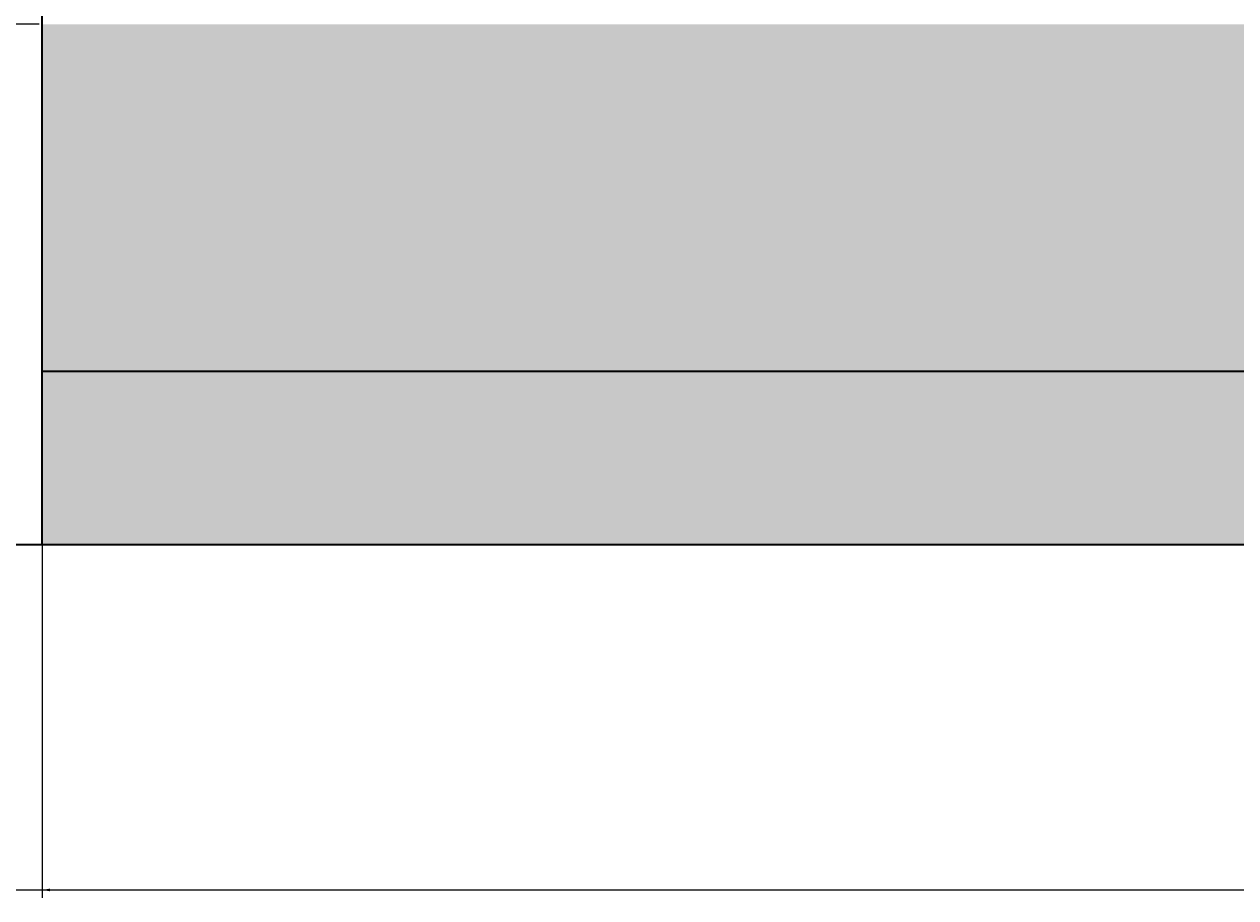
# Model space of a CAD drawing. Units: inches. Extents: x 4508 to 4723, y 847 to 1020.
# Tile 2 of 32: x 4550 to 4577, y 867 to 887. Entities that reach past the tile are written whole.
import ezdxf

# ---------------------------------------------------------------- set-up
doc = ezdxf.new("R2010")
doc.units = ezdxf.units.IN
for name, color, linetype, lineweight in [('A-ANNO-DIMS', 2, 'Continuous', 18), ('A-WALL', 7, 'Continuous', 35), ('A-WALL-PATT', 254, 'Continuous', 13)]:
    doc.layers.add(name, color=color, linetype=linetype, lineweight=lineweight)
doc.styles.get("Standard").update_dxf_attribs({"font": 'arial.ttf'})
doc.dimstyles.get("Standard").update_dxf_attribs({"dimtxt": 0.18, "dimasz": 0.18, "dimexe": 0.18, "dimexo": 0.0625, "dimgap": 0.09, "dimtad": 0, "dimtih": 1, "dimtoh": 1, "dimdec": 4, "dimzin": 0, "dimdsep": 46, "dimtxsty": 'Standard', "dimcen": 0.09, "dimadec": 0, "dimazin": 0, "dimtfac": 1, "dimtdec": 4, "dimtofl": 0, "dimtmove": 0, "dimatfit": 3, "dimfxl": 1, "dimtolj": 1, "dimtzin": 0, "dimarcsym": 0})

# ---------------------------------------------------------------- blocks, each defined once
blk = doc.blocks.new('*D2')
at = {"layer": 'A-ANNO-DIMS', "color": 0, "lineweight": -2, "transparency": 16777216}
for p, q in [((4540.994, 874.684), (4540.994, 866.617)), ((4693.994, 874.684), (4693.994, 866.617)), ((4541.174, 866.797), (4617.213, 866.797)), ((4693.814, 866.797), (4617.774, 866.797))]:
    blk.add_line(p, q, dxfattribs=at)
at = {"layer": 'A-ANNO-DIMS', "color": 0, "lineweight": 9, "transparency": 16777216}
for points in [[(4541.174, 866.827), (4541.174, 866.767), (4540.994, 866.797)], [(4693.814, 866.827), (4693.814, 866.767), (4693.994, 866.797)]]:
    blk.add_solid(points, dxfattribs=at)
at = {"layer": 'Defpoints', "color": 0, "lineweight": 9, "transparency": 16777216}
for p in [(4540.994, 874.747), (4693.994, 874.747), (4693.994, 866.797)]:
    blk.add_point(p, dxfattribs=at)
at = {"layer": 'A-ANNO-DIMS', "color": 0, "transparency": 16777216, "insert": (4617.494, 866.797), "char_height": 0.18, "attachment_point": 5}
blk.add_mtext('\\A1;153', dxfattribs=at)
blk = doc.blocks.new('*D14')
at = {"layer": 'A-ANNO-DIMS', "color": 0, "lineweight": -2, "transparency": 16777216}
for p, q in [((4549.931, 886.747), (4532.864, 886.747)), ((4533.044, 886.567), (4533.044, 880.927)), ((4533.044, 874.927), (4533.044, 880.567)), ((4549.931, 874.747), (4532.864, 874.747))]:
    blk.add_line(p, q, dxfattribs=at)
at = {"layer": 'A-ANNO-DIMS', "color": 0, "lineweight": 9, "transparency": 16777216}
for points in [[(4533.014, 886.567), (4533.074, 886.567), (4533.044, 886.747)], [(4533.014, 874.927), (4533.074, 874.927), (4533.044, 874.747)]]:
    blk.add_solid(points, dxfattribs=at)
at = {"layer": 'Defpoints', "color": 0, "lineweight": 9, "transparency": 16777216}
for p in [(4533.044, 886.747), (4549.994, 886.747), (4549.994, 874.747)]:
    blk.add_point(p, dxfattribs=at)
at = {"layer": 'A-ANNO-DIMS', "color": 0, "transparency": 16777216, "insert": (4533.044, 880.747), "char_height": 0.18, "attachment_point": 5}
blk.add_mtext('\\A1;12', dxfattribs=at)
blk = doc.blocks.new('*D24')
at = {"layer": 'A-ANNO-DIMS', "color": 0, "lineweight": -2, "transparency": 16777216}
for p, q in [((4549.994, 886.684), (4549.994, 866.617)), ((4657.994, 886.684), (4657.994, 866.617)), ((4550.174, 866.797), (4603.713, 866.797)), ((4657.814, 866.797), (4604.274, 866.797))]:
    blk.add_line(p, q, dxfattribs=at)
at = {"layer": 'A-ANNO-DIMS', "color": 0, "lineweight": 9, "transparency": 16777216}
for points in [[(4550.174, 866.827), (4550.174, 866.767), (4549.994, 866.797)], [(4657.814, 866.827), (4657.814, 866.767), (4657.994, 866.797)]]:
    blk.add_solid(points, dxfattribs=at)
at = {"layer": 'Defpoints', "color": 0, "lineweight": 9, "transparency": 16777216}
for p in [(4549.994, 886.747), (4657.994, 886.747), (4657.994, 866.797)]:
    blk.add_point(p, dxfattribs=at)
at = {"layer": 'A-ANNO-DIMS', "color": 0, "transparency": 16777216, "insert": (4603.994, 866.797), "char_height": 0.18, "attachment_point": 5}
blk.add_mtext('\\A1;108', dxfattribs=at)

msp = doc.modelspace()

# ---------------------------------------------------------------- hatches: boundary and pattern name
at = {"layer": 'A-WALL-PATT', "transparency": 33554508}
h = msp.add_hatch(color=256, dxfattribs=at)
h.dxf.hatch_style = 1
h.paths.add_polyline_path([(4661.6706, 954.043, -0.3739004), (4658.5765, 957.6021, -1), (4665.7646, 957.6021, -0.3739004), (4662.6706, 954.043), (4662.6706, 944.4021, -0.2114781), (4670.3062, 945.0869), (4670.3062, 968.0592, -0.4632086), (4663.3246, 973.9783, -0.4632086), (4670.3062, 979.8975), (4670.3062, 994.7469), (4588.9938, 994.7469), (4588.9938, 904.7469), (4657.9938, 904.7469), (4657.9938, 886.7469), (4549.9938, 886.7469), (4549.9938, 878.7469), (4693.9938, 878.7469), (4693.9938, 994.7469), (4671.8062, 994.7469), (4671.8062, 979.4411, -0.2941682), (4675.3246, 973.9783, -0.2941682), (4671.8062, 968.5156), (4671.8062, 944.4278, -0.2741114), (4676.7298, 936.1217, -0.2741114), (4671.8062, 927.8155), (4671.8062, 907.6998, -0.3779645), (4677.0562, 901.7469, -0.3779645), (4671.8062, 895.7939), (4671.8062, 883.7469), (4670.3062, 883.7469), (4670.3062, 895.7939, -0.3779645), (4665.0562, 901.7469, -0.3779645), (4670.3062, 907.6998), (4670.3062, 927.1564, -0.2114781), (4662.6706, 927.8412), (4662.6706, 918.2003, -0.3739004), (4665.7646, 914.6412, -1), (4658.5765, 914.6412, -0.3739004), (4661.6706, 918.2003), (4661.6706, 928.4807, -0.2391825), (4657.7936, 936.1217, -0.2391825), (4661.6706, 943.7626)])
at = {"layer": 'A-WALL-PATT', "transparency": 33554556}
h = msp.add_hatch(color=256, dxfattribs=at)
h.dxf.hatch_style = 1
h.paths.add_polyline_path([(4689.9938, 878.7469), (4549.9938, 878.7469), (4549.9938, 874.7469), (4689.9938, 874.7469)])

# ---------------------------------------------------------------- linework, layer by layer
at = {"layer": 'A-WALL'}
for p, q in [((4549.9938, 874.7469), (4549.9938, 994.7469)), ((4693.9938, 878.7469), (4549.9938, 878.7469)), ((4549.9938, 874.7469), (4540.9938, 874.7469)), ((4693.9938, 874.7469), (4549.9938, 874.7469))]:
    msp.add_line(p, q, dxfattribs=at)

# ---------------------------------------------------------------- dimensions: what is measured, and where the dimension line sits
at = {"layer": 'A-ANNO-DIMS'}
dim = msp.add_linear_dim(base=(4533.0438, 886.7469), p1=(4549.9938, 874.7469), p2=(4549.9938, 886.7469), angle=90, dimstyle='Standard', override={"dimdec": 0, "dimlfac": 1, "dimrnd": 0, "dimzin": 0, "dimdsep": 46, "dimlunit": 2}, dxfattribs=at)
dim.commit()
dim.dimension.update_dxf_attribs({"geometry": '*D14', "text_midpoint": (4533.0438, 880.7469)})
for base, p1, p2, picture, middle in [((4657.9938, 866.7969), (4549.9938, 886.7469), (4657.9938, 886.7469), '*D24', (4603.9938, 866.7969)), ((4693.9938, 866.7969), (4540.9938, 874.7469), (4693.9938, 874.7469), '*D2', (4617.4938, 866.7969))]:
    dim = msp.add_linear_dim(base=base, p1=p1, p2=p2, dimstyle='Standard', override={"dimdec": 0, "dimlfac": 1, "dimrnd": 0, "dimzin": 0, "dimdsep": 46, "dimlunit": 2}, dxfattribs=at)
    dim.commit()
    dim.dimension.update_dxf_attribs({"geometry": picture, "text_midpoint": middle})

doc.saveas('drawing.dxf')
